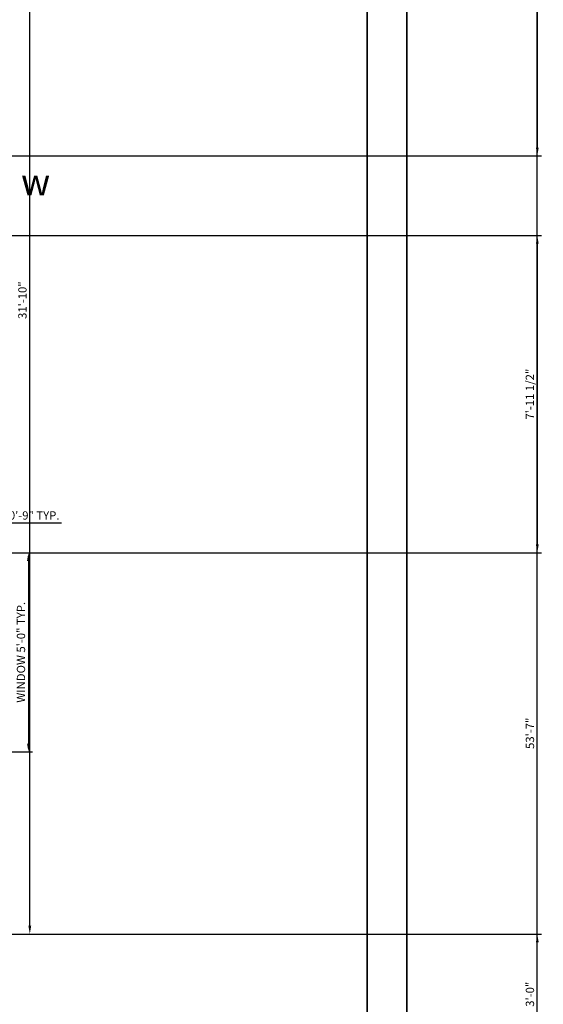
# Model space of a CAD drawing. Units: inches. Extents: x 2901 to 5923, y 918 to 2827.
# Tile 13 of 16: x 4898 to 5056, y 1227 to 1524. Entities that reach past the tile are written whole.
import ezdxf

# ---------------------------------------------------------------- set-up
doc = ezdxf.new("R2010")
doc.units = ezdxf.units.IN
for name, color, linetype, lineweight in [('A-ANNO-DIMS', 2, 'Continuous', 18), ('A-ANNO-TEXT', 7, 'Continuous', 18), ('C-PROP', 7, 'Continuous', 35)]:
    doc.layers.add(name, color=color, linetype=linetype, lineweight=lineweight)
doc.styles.get("Standard").update_dxf_attribs({"font": 'arial.ttf'})
doc.dimstyles.new('Copy of ISO-25', dxfattribs={"dimtxt": 2.5, "dimasz": 2.5, "dimexe": 1.25, "dimexo": 0.625, "dimtad": 1, "dimdec": 1, "dimlunit": 4, "dimtxsty": 'Standard', "dimcen": 2.5, "dimadec": 0, "dimazin": 0, "dimtfac": 1, "dimtdec": 1, "dimtmove": 0, "dimatfit": 3, "dimfxl": 1, "dimarcsym": 0})

# ---------------------------------------------------------------- blocks, each defined once
blk = doc.blocks.new('*D35')
at = {"layer": 'A-ANNO-DIMS', "color": 0, "lineweight": -2, "transparency": 16777216}
for p, q in [((4892.69, 1630.4), (4902.74, 1630.4)), ((4901.49, 1250.9), (4901.49, 1627.9)), ((4892.69, 1248.4), (4902.74, 1248.4))]:
    blk.add_line(p, q, dxfattribs=at)
at = {"layer": 'A-ANNO-DIMS', "color": 0, "transparency": 16777216}
for points in [[(4901.07, 1627.9), (4901.91, 1627.9), (4901.49, 1630.4)], [(4901.07, 1250.9), (4901.91, 1250.9), (4901.49, 1248.4)]]:
    blk.add_solid(points, dxfattribs=at)
at = {"layer": 'Defpoints', "color": 0, "transparency": 16777216}
for p in [(4892.07, 1630.4), (4901.49, 1630.4), (4892.07, 1248.4)]:
    blk.add_point(p, dxfattribs=at)
at = {"layer": 'A-ANNO-DIMS', "color": 0, "transparency": 16777216, "insert": (4899.59, 1439.4), "char_height": 2.5, "attachment_point": 5, "rotation": 90}
blk.add_mtext('31\'-10"', dxfattribs=at)
blk = doc.blocks.new('*D73')
at = {"layer": 'A-ANNO-DIMS', "color": 0, "lineweight": -2, "transparency": 16777216}
for p, q in [((4892.69, 1363.31), (4902.32, 1363.31)), ((4901.07, 1360.81), (4901.07, 1305.81)), ((4892.69, 1303.31), (4902.32, 1303.31))]:
    blk.add_line(p, q, dxfattribs=at)
at = {"layer": 'A-ANNO-DIMS', "color": 0, "transparency": 16777216}
for points in [[(4900.65, 1360.81), (4901.49, 1360.81), (4901.07, 1363.31)], [(4900.65, 1305.81), (4901.49, 1305.81), (4901.07, 1303.31)]]:
    blk.add_solid(points, dxfattribs=at)
at = {"layer": 'Defpoints', "color": 0, "transparency": 16777216}
for p in [(4892.07, 1363.31), (4892.07, 1303.31), (4901.07, 1303.31)]:
    blk.add_point(p, dxfattribs=at)
at = {"layer": 'A-ANNO-DIMS', "color": 0, "transparency": 16777216, "insert": (4899.15, 1333.31), "char_height": 2.5, "attachment_point": 5, "rotation": 90}
blk.add_mtext('WINDOW 5\'-0" TYP.', dxfattribs=at)
blk = doc.blocks.new('*D74')
at = {"layer": 'A-ANNO-DIMS', "color": 0, "lineweight": -2, "transparency": 16777216}
for p, q in [((4883.07, 1363.93), (4883.07, 1373.56)), ((4892.07, 1363.93), (4892.07, 1373.56)), ((4885.57, 1372.31), (4889.57, 1372.31)), ((4892.07, 1372.31), (4911.06, 1372.31))]:
    blk.add_line(p, q, dxfattribs=at)
at = {"layer": 'A-ANNO-DIMS', "color": 0, "transparency": 16777216}
for points in [[(4885.57, 1372.72), (4885.57, 1371.89), (4883.07, 1372.31)], [(4889.57, 1372.72), (4889.57, 1371.89), (4892.07, 1372.31)]]:
    blk.add_solid(points, dxfattribs=at)
at = {"layer": 'Defpoints', "color": 0, "transparency": 16777216}
for p in [(4892.07, 1372.31), (4883.07, 1363.31), (4892.07, 1363.31)]:
    blk.add_point(p, dxfattribs=at)
at = {"layer": 'A-ANNO-DIMS', "color": 0, "transparency": 16777216, "insert": (4902.81, 1374.21), "char_height": 2.5, "attachment_point": 5}
blk.add_mtext('0\'-9" TYP.', dxfattribs=at)
blk = doc.blocks.new('*D89')
at = {"layer": 'A-ANNO-DIMS', "color": 0, "lineweight": -2, "transparency": 16777216}
for p, q in [((4892.69, 1630.4), (5055.73, 1630.4)), ((5054.48, 989.9), (5054.48, 1627.9)), ((4709.69, 987.4), (5055.73, 987.4))]:
    blk.add_line(p, q, dxfattribs=at)
at = {"layer": 'A-ANNO-DIMS', "color": 0, "transparency": 16777216}
for points in [[(5054.06, 1627.9), (5054.9, 1627.9), (5054.48, 1630.4)], [(5054.06, 989.9), (5054.9, 989.9), (5054.48, 987.4)]]:
    blk.add_solid(points, dxfattribs=at)
at = {"layer": 'Defpoints', "color": 0, "transparency": 16777216}
for p in [(4892.07, 1630.4), (5054.48, 1630.4), (4709.07, 987.4)]:
    blk.add_point(p, dxfattribs=at)
at = {"layer": 'A-ANNO-DIMS', "color": 0, "transparency": 16777216, "insert": (5052.58, 1308.9), "char_height": 2.5, "attachment_point": 5, "rotation": 90}
blk.add_mtext('53\'-7"', dxfattribs=at)
blk = doc.blocks.new('*D96')
at = {"layer": 'A-ANNO-DIMS', "color": 0, "lineweight": -2, "transparency": 16777216}
for p, q in [((4892.69, 1630.4), (5055.73, 1630.4)), ((5054.48, 1627.9), (5054.48, 1485.37)), ((4892.69, 1482.87), (5055.73, 1482.87))]:
    blk.add_line(p, q, dxfattribs=at)
at = {"layer": 'A-ANNO-DIMS', "color": 0, "transparency": 16777216}
for points in [[(5054.06, 1627.9), (5054.9, 1627.9), (5054.48, 1630.4)], [(5054.06, 1485.37), (5054.9, 1485.37), (5054.48, 1482.87)]]:
    blk.add_solid(points, dxfattribs=at)
at = {"layer": 'Defpoints', "color": 0, "transparency": 16777216}
for p in [(4892.07, 1630.4), (4892.07, 1482.87), (5054.48, 1482.87)]:
    blk.add_point(p, dxfattribs=at)
at = {"layer": 'A-ANNO-DIMS', "color": 0, "transparency": 16777216, "insert": (5052.56, 1556.63), "char_height": 2.5, "attachment_point": 5, "rotation": 90}
blk.add_mtext('12\'-3 1/2"', dxfattribs=at)
blk = doc.blocks.new('*D97')
at = {"layer": 'A-ANNO-DIMS', "color": 0, "lineweight": -2, "transparency": 16777216}
for p, q in [((4892.69, 1458.87), (5055.73, 1458.87)), ((5054.48, 1456.37), (5054.48, 1365.81)), ((4892.69, 1363.31), (5055.73, 1363.31))]:
    blk.add_line(p, q, dxfattribs=at)
at = {"layer": 'A-ANNO-DIMS', "color": 0, "transparency": 16777216}
for points in [[(5054.06, 1456.37), (5054.9, 1456.37), (5054.48, 1458.87)], [(5054.06, 1365.81), (5054.9, 1365.81), (5054.48, 1363.31)]]:
    blk.add_solid(points, dxfattribs=at)
at = {"layer": 'Defpoints', "color": 0, "transparency": 16777216}
for p in [(4892.07, 1458.87), (4892.07, 1363.31), (5054.48, 1363.31)]:
    blk.add_point(p, dxfattribs=at)
at = {"layer": 'A-ANNO-DIMS', "color": 0, "transparency": 16777216, "insert": (5052.56, 1411.09), "char_height": 2.5, "attachment_point": 5, "rotation": 90}
blk.add_mtext('7\'-11 1/2"', dxfattribs=at)
blk = doc.blocks.new('*D99')
at = {"layer": 'A-ANNO-DIMS', "color": 0, "lineweight": -2, "transparency": 16777216}
for p, q in [((4820.69, 1248.4), (5055.73, 1248.4)), ((5054.48, 1214.66), (5054.48, 1245.9)), ((4820.69, 1212.16), (5055.73, 1212.16))]:
    blk.add_line(p, q, dxfattribs=at)
at = {"layer": 'A-ANNO-DIMS', "color": 0, "transparency": 16777216}
for points in [[(5054.06, 1245.9), (5054.9, 1245.9), (5054.48, 1248.4)], [(5054.06, 1214.66), (5054.9, 1214.66), (5054.48, 1212.16)]]:
    blk.add_solid(points, dxfattribs=at)
at = {"layer": 'Defpoints', "color": 0, "transparency": 16777216}
for p in [(4820.07, 1248.4), (5054.48, 1248.4), (4820.07, 1212.16)]:
    blk.add_point(p, dxfattribs=at)
at = {"layer": 'A-ANNO-DIMS', "color": 0, "transparency": 16777216, "insert": (5052.58, 1230.28), "char_height": 2.5, "attachment_point": 5, "rotation": 90}
blk.add_mtext('3\'-0"', dxfattribs=at)

msp = doc.modelspace()

# ---------------------------------------------------------------- linework, layer by layer
at = {"layer": 'C-PROP'}
msp.add_lwpolyline([(4288.18, 1684.29), (5015.18, 1684.29), (5015.18, 958.29), (4288.18, 958.29)], close=True, dxfattribs=at)
msp.add_lwpolyline([(5003.18, 978.26), (5003.18, 970.29), (4300.18, 970.29), (4300.18, 1672.29), (5003.18, 1672.29), (5003.18, 1132.27)], dxfattribs=at)

# ---------------------------------------------------------------- texts
at = {"layer": 'A-ANNO-TEXT'}
msp.add_text('w', height=8, dxfattribs=at).set_placement((4898.86, 1470.95))

# ---------------------------------------------------------------- dimensions: what is measured, and where the dimension line sits
at = {"layer": 'A-ANNO-DIMS'}
for base, p1, p2, override, picture, middle in [((5054.48, 1630.4), (4709.07, 987.4), (4892.07, 1630.4), {"dimdec": 1, "dimlfac": 1, "dimrnd": 0, "dimzin": 1, "dimdsep": 46, "dimlunit": 4, "dimfrac": 2}, '*D89', (5052.58, 1308.9)), ((4901.49, 1630.4), (4892.07, 1248.4), (4892.07, 1630.4), {"dimclrd": 0, "dimclre": 0, "dimclrt": 0}, '*D35', (4899.59, 1439.4)), ((5054.48, 1482.87), (4892.07, 1630.4), (4892.07, 1482.87), {"dimdec": 1, "dimlfac": 1, "dimrnd": 0, "dimzin": 1, "dimdsep": 46, "dimlunit": 4, "dimfrac": 2}, '*D96', (5052.56, 1556.63)), ((5054.48, 1363.31), (4892.07, 1458.87), (4892.07, 1363.31), {"dimdec": 1, "dimlfac": 1, "dimrnd": 0, "dimzin": 1, "dimdsep": 46, "dimlunit": 4, "dimfrac": 2}, '*D97', (5052.56, 1411.09)), ((5054.48, 1248.4), (4820.07, 1212.16), (4820.07, 1248.4), {"dimdec": 1, "dimlfac": 1, "dimrnd": 0, "dimzin": 1, "dimdsep": 46, "dimlunit": 4, "dimfrac": 2}, '*D99', (5052.58, 1230.28))]:
    dim = msp.add_linear_dim(base=base, p1=p1, p2=p2, angle=90, dimstyle='Copy of ISO-25', override=override, dxfattribs=at)
    dim.commit()
    dim.dimension.update_dxf_attribs({"geometry": picture, "text_midpoint": middle})
dim = msp.add_linear_dim(base=(4892.07, 1372.31), p1=(4883.07, 1363.31), p2=(4892.07, 1363.31), text='<> TYP.', dimstyle='Copy of ISO-25', override={"dimdec": 1, "dimlfac": 1, "dimrnd": 0, "dimzin": 1, "dimdsep": 46, "dimlunit": 4, "dimfrac": 2}, dxfattribs=at)
dim.commit()
dim.dimension.update_dxf_attribs({"geometry": '*D74', "text_midpoint": (4902.81, 1374.21)})
dim = msp.add_linear_dim(base=(4901.07, 1303.31), p1=(4892.07, 1363.31), p2=(4892.07, 1303.31), angle=270, text='WINDOW <> TYP.', dimstyle='Copy of ISO-25', override={"dimdec": 1, "dimlfac": 1, "dimrnd": 0, "dimzin": 1, "dimdsep": 46, "dimlunit": 4, "dimfrac": 2}, dxfattribs=at)
dim.commit()
dim.dimension.update_dxf_attribs({"geometry": '*D73', "text_midpoint": (4899.15, 1333.31)})

doc.saveas('drawing.dxf')
